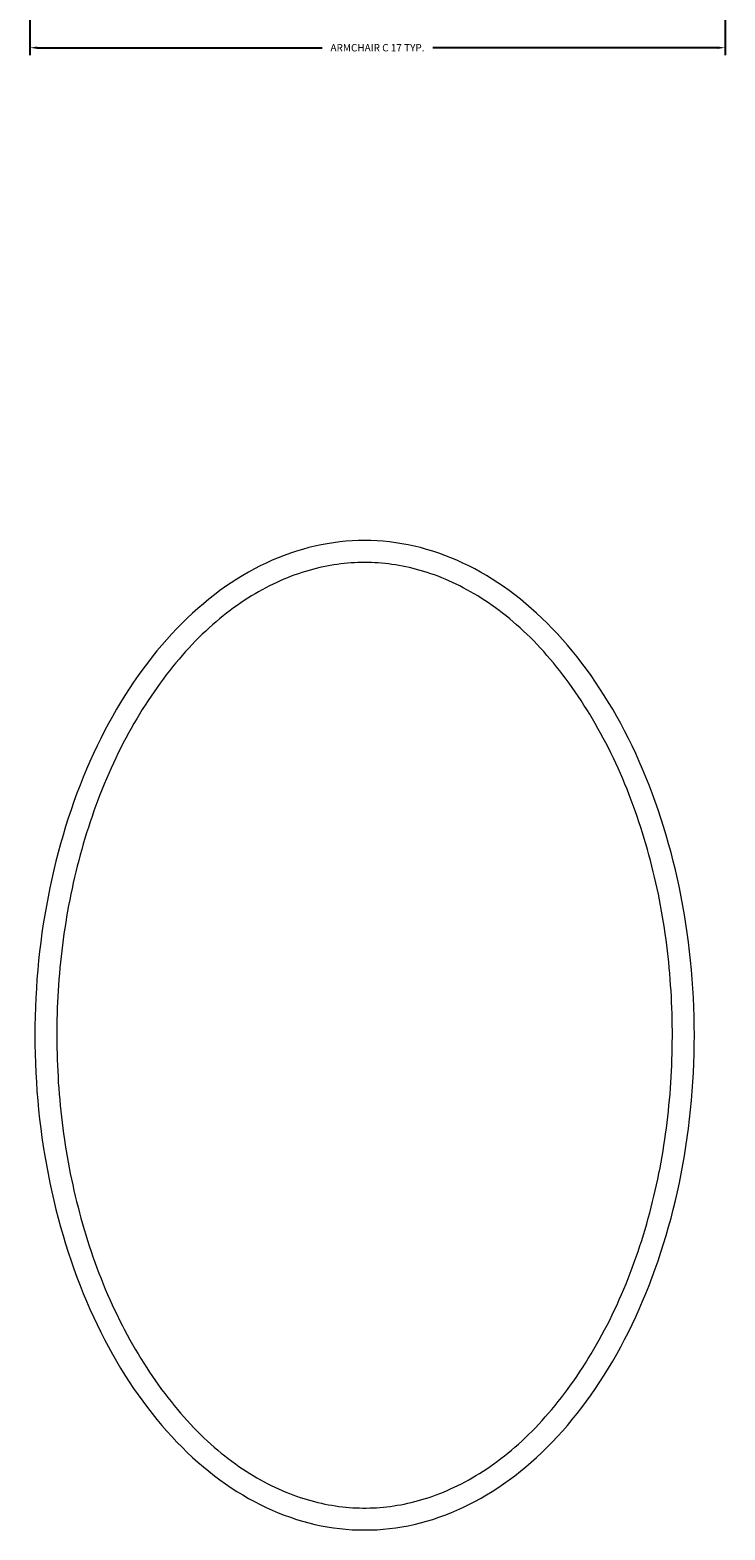
# Model space of a CAD drawing. Units: inches. Extents: x 963 to 2075, y 289 to 2657.
# Tile 22 of 98: x 1467 to 1484, y 1764 to 1800. Entities that reach past the tile are written whole.
import ezdxf

# ---------------------------------------------------------------- set-up
doc = ezdxf.new("R2010")
doc.units = ezdxf.units.IN
doc.layers.add('A-ANNO-DIMS', color=2, linetype='Continuous', lineweight=18)
doc.layers.add('A-FURN', color=8, linetype='Continuous', lineweight=18)
doc.styles.get("Standard").update_dxf_attribs({"font": 'arial.ttf'})
doc.dimstyles.get("Standard").update_dxf_attribs({"dimtxt": 0.18, "dimasz": 0.18, "dimexe": 0.18, "dimexo": 0.0625, "dimgap": 0.09, "dimtad": 0, "dimtih": 1, "dimtoh": 1, "dimdec": 4, "dimzin": 0, "dimdsep": 46, "dimtxsty": 'Standard', "dimcen": 0.09, "dimadec": 0, "dimazin": 0, "dimtfac": 1, "dimtdec": 4, "dimtofl": 0, "dimtmove": 0, "dimatfit": 3, "dimfxl": 1, "dimtolj": 1, "dimtzin": 0, "dimarcsym": 0})

# ---------------------------------------------------------------- blocks, each defined once
blk = doc.blocks.new('TABLE-OVAL')
at = {"ltscale": 0.03}
blk.add_polyline3d([(7.656, -0.197, 0), (7.809, -0.194, 0), (7.963, -0.188, 0), (8.116, -0.177, 0), (8.269, -0.162, 0), (8.422, -0.142, 0), (8.575, -0.118, 0), (8.727, -0.09, 0), (8.879, -0.057, 0), (9.031, -0.021, 0), (9.182, 0.021, 0), (9.332, 0.066, 0), (9.482, 0.116, 0), (9.632, 0.17, 0), (9.78, 0.228, 0), (9.928, 0.29, 0), (10.075, 0.357, 0), (10.221, 0.428, 0), (10.366, 0.503, 0), (10.51, 0.582, 0), (10.653, 0.665, 0), (10.796, 0.752, 0), (10.937, 0.843, 0), (11.076, 0.938, 0), (11.215, 1.037, 0), (11.352, 1.14, 0), (11.488, 1.247, 0), (11.623, 1.358, 0), (11.756, 1.472, 0), (11.888, 1.59, 0), (12.018, 1.712, 0), (12.147, 1.838, 0), (12.274, 1.967, 0), (12.399, 2.1, 0), (12.523, 2.237, 0), (12.645, 2.376, 0), (12.765, 2.52, 0), (12.883, 2.666, 0), (13, 2.817, 0), (13.114, 2.97, 0), (13.227, 3.126, 0), (13.337, 3.286, 0), (13.446, 3.449, 0), (13.552, 3.615, 0), (13.657, 3.784, 0), (13.759, 3.955, 0), (13.859, 4.13, 0), (13.957, 4.308, 0), (14.052, 4.488, 0), (14.145, 4.671, 0), (14.236, 4.856, 0), (14.325, 5.044, 0), (14.411, 5.235, 0), (14.495, 5.428, 0), (14.576, 5.623, 0), (14.655, 5.821, 0), (14.731, 6.021, 0), (14.805, 6.222, 0), (14.877, 6.426, 0), (14.945, 6.632, 0), (15.011, 6.84, 0), (15.075, 7.05, 0), (15.135, 7.261, 0), (15.193, 7.475, 0), (15.249, 7.689, 0), (15.301, 7.906, 0), (15.351, 8.123, 0), (15.399, 8.343, 0), (15.443, 8.563, 0), (15.485, 8.785, 0), (15.523, 9.007, 0), (15.559, 9.231, 0), (15.592, 9.456, 0), (15.623, 9.682, 0), (15.65, 9.908, 0), (15.675, 10.136, 0), (15.697, 10.364, 0), (15.715, 10.592, 0), (15.731, 10.821, 0), (15.744, 11.051, 0), (15.755, 11.28, 0), (15.762, 11.51, 0), (15.766, 11.741, 0), (15.768, 11.971, 0), (15.766, 12.201, 0), (15.762, 12.431, 0), (15.755, 12.661, 0), (15.744, 12.891, 0), (15.731, 13.12, 0), (15.715, 13.349, 0), (15.697, 13.578, 0), (15.675, 13.806, 0), (15.65, 14.033, 0), (15.623, 14.26, 0), (15.592, 14.486, 0), (15.559, 14.71, 0), (15.523, 14.934, 0), (15.485, 15.157, 0), (15.443, 15.379, 0), (15.399, 15.599, 0), (15.351, 15.818, 0), (15.301, 16.036, 0), (15.249, 16.252, 0), (15.193, 16.467, 0), (15.135, 16.68, 0), (15.075, 16.892, 0), (15.011, 17.101, 0), (14.945, 17.309, 0), (14.877, 17.515, 0), (14.805, 17.719, 0), (14.731, 17.921, 0), (14.655, 18.121, 0), (14.576, 18.318, 0), (14.495, 18.514, 0), (14.411, 18.707, 0), (14.325, 18.897, 0), (14.236, 19.085, 0), (14.145, 19.271, 0), (14.052, 19.454, 0), (13.957, 19.634, 0), (13.859, 19.811, 0), (13.759, 19.986, 0), (13.657, 20.158, 0), (13.552, 20.327, 0), (13.446, 20.493, 0), (13.337, 20.656, 0), (13.227, 20.815, 0), (13.114, 20.972, 0), (13, 21.125, 0), (12.883, 21.275, 0), (12.765, 21.422, 0), (12.645, 21.565, 0), (12.523, 21.705, 0), (12.399, 21.842, 0), (12.274, 21.974, 0), (12.147, 22.104, 0), (12.018, 22.229, 0), (11.888, 22.351, 0), (11.756, 22.47, 0), (11.623, 22.584, 0), (11.488, 22.695, 0), (11.352, 22.802, 0), (11.215, 22.905, 0), (11.076, 23.004, 0), (10.937, 23.099, 0), (10.796, 23.19, 0), (10.653, 23.277, 0), (10.51, 23.36, 0), (10.366, 23.439, 0), (10.221, 23.514, 0), (10.075, 23.585, 0), (9.928, 23.651, 0), (9.78, 23.714, 0), (9.632, 23.772, 0), (9.482, 23.826, 0), (9.332, 23.876, 0), (9.182, 23.921, 0), (9.031, 23.962, 0), (8.879, 23.999, 0), (8.727, 24.032, 0), (8.575, 24.06, 0), (8.422, 24.084, 0), (8.269, 24.103, 0), (8.116, 24.119, 0), (7.963, 24.13, 0), (7.809, 24.136, 0), (7.656, 24.138, 0), (7.502, 24.136, 0), (7.349, 24.13, 0), (7.196, 24.119, 0), (7.042, 24.103, 0), (6.89, 24.084, 0), (6.737, 24.06, 0), (6.585, 24.032, 0), (6.433, 23.999, 0), (6.281, 23.962, 0), (6.13, 23.921, 0), (5.979, 23.876, 0), (5.83, 23.826, 0), (5.68, 23.772, 0), (5.532, 23.714, 0), (5.384, 23.651, 0), (5.237, 23.585, 0), (5.091, 23.514, 0), (4.946, 23.439, 0), (4.802, 23.36, 0), (4.658, 23.277, 0), (4.516, 23.19, 0), (4.375, 23.099, 0), (4.236, 23.004, 0), (4.097, 22.905, 0), (3.96, 22.802, 0), (3.824, 22.695, 0), (3.689, 22.584, 0), (3.556, 22.47, 0), (3.424, 22.351, 0), (3.294, 22.229, 0), (3.165, 22.104, 0), (3.038, 21.974, 0), (2.913, 21.842, 0), (2.789, 21.705, 0), (2.667, 21.565, 0), (2.547, 21.422, 0), (2.429, 21.275, 0), (2.312, 21.125, 0), (2.198, 20.972, 0), (2.085, 20.815, 0), (1.975, 20.656, 0), (1.866, 20.493, 0), (1.76, 20.327, 0), (1.655, 20.158, 0), (1.553, 19.986, 0), (1.453, 19.811, 0), (1.355, 19.634, 0), (1.26, 19.454, 0), (1.166, 19.271, 0), (1.076, 19.085, 0), (0.987, 18.897, 0), (0.901, 18.707, 0), (0.817, 18.514, 0), (0.736, 18.318, 0), (0.657, 18.121, 0), (0.58, 17.921, 0), (0.507, 17.719, 0), (0.435, 17.515, 0), (0.367, 17.309, 0), (0.301, 17.101, 0), (0.237, 16.892, 0), (0.177, 16.68, 0), (0.118, 16.467, 0), (0.063, 16.252, 0), (0.01, 16.036, 0), (-0.039, 15.818, 0), (-0.087, 15.599, 0), (-0.131, 15.379, 0), (-0.173, 15.157, 0), (-0.211, 14.934, 0), (-0.247, 14.71, 0), (-0.281, 14.486, 0), (-0.311, 14.26, 0), (-0.338, 14.033, 0), (-0.363, 13.806, 0), (-0.385, 13.578, 0), (-0.403, 13.349, 0), (-0.419, 13.12, 0), (-0.432, 12.891, 0), (-0.443, 12.661, 0), (-0.45, 12.431, 0), (-0.454, 12.201, 0), (-0.456, 11.971, 0), (-0.454, 11.741, 0), (-0.45, 11.51, 0), (-0.443, 11.28, 0), (-0.432, 11.051, 0), (-0.419, 10.821, 0), (-0.403, 10.592, 0), (-0.385, 10.364, 0), (-0.363, 10.136, 0), (-0.338, 9.908, 0), (-0.311, 9.682, 0), (-0.281, 9.456, 0), (-0.247, 9.231, 0), (-0.211, 9.007, 0), (-0.173, 8.785, 0), (-0.131, 8.563, 0), (-0.087, 8.343, 0), (-0.039, 8.123, 0), (0.01, 7.906, 0), (0.063, 7.689, 0), (0.118, 7.475, 0), (0.177, 7.261, 0), (0.237, 7.05, 0), (0.301, 6.84, 0), (0.367, 6.632, 0), (0.435, 6.426, 0), (0.507, 6.222, 0), (0.58, 6.021, 0), (0.657, 5.821, 0), (0.736, 5.623, 0), (0.817, 5.428, 0), (0.901, 5.235, 0), (0.987, 5.044, 0), (1.076, 4.856, 0), (1.166, 4.671, 0), (1.26, 4.488, 0), (1.355, 4.308, 0), (1.453, 4.13, 0), (1.553, 3.955, 0), (1.655, 3.784, 0), (1.76, 3.615, 0), (1.866, 3.449, 0), (1.975, 3.286, 0), (2.085, 3.126, 0), (2.198, 2.97, 0), (2.312, 2.817, 0), (2.429, 2.666, 0), (2.547, 2.52, 0), (2.667, 2.376, 0), (2.789, 2.237, 0), (2.913, 2.1, 0), (3.038, 1.967, 0), (3.165, 1.838, 0), (3.294, 1.712, 0), (3.424, 1.59, 0), (3.556, 1.472, 0), (3.689, 1.358, 0), (3.824, 1.247, 0), (3.96, 1.14, 0), (4.097, 1.037, 0), (4.236, 0.938, 0), (4.375, 0.843, 0), (4.516, 0.752, 0), (4.658, 0.665, 0), (4.802, 0.582, 0), (4.946, 0.503, 0), (5.091, 0.428, 0), (5.237, 0.357, 0), (5.384, 0.29, 0), (5.532, 0.228, 0), (5.68, 0.17, 0), (5.83, 0.116, 0), (5.979, 0.066, 0), (6.13, 0.021, 0), (6.281, -0.021, 0), (6.433, -0.057, 0), (6.585, -0.09, 0), (6.737, -0.118, 0), (6.89, -0.142, 0), (7.042, -0.162, 0), (7.196, -0.177, 0), (7.349, -0.188, 0), (7.502, -0.194, 0), (7.656, -0.197, 0)], dxfattribs=at)
blk.add_polyline3d([(7.656, 0.344, 0), (7.739, 0.345, 0), (7.822, 0.347, 0), (7.906, 0.351, 0), (7.99, 0.356, 0), (8.074, 0.362, 0), (8.159, 0.37, 0), (8.244, 0.38, 0), (8.33, 0.391, 0), (8.415, 0.404, 0), (8.501, 0.418, 0), (8.588, 0.434, 0), (8.674, 0.451, 0), (8.761, 0.47, 0), (8.848, 0.491, 0), (8.935, 0.513, 0), (9.023, 0.538, 0), (9.11, 0.563, 0), (9.198, 0.591, 0), (9.286, 0.62, 0), (9.375, 0.651, 0), (9.463, 0.684, 0), (9.552, 0.719, 0), (9.64, 0.755, 0), (9.729, 0.794, 0), (9.818, 0.834, 0), (9.907, 0.876, 0), (9.995, 0.92, 0), (10.084, 0.966, 0), (10.173, 1.013, 0), (10.262, 1.063, 0), (10.35, 1.114, 0), (10.439, 1.167, 0), (10.527, 1.222, 0), (10.615, 1.279, 0), (10.703, 1.338, 0), (10.791, 1.398, 0), (10.878, 1.461, 0), (10.965, 1.525, 0), (11.052, 1.592, 0), (11.139, 1.66, 0), (11.225, 1.73, 0), (11.311, 1.802, 0), (11.396, 1.876, 0), (11.481, 1.952, 0), (11.565, 2.03, 0), (11.649, 2.109, 0), (11.733, 2.191, 0), (11.815, 2.275, 0), (11.898, 2.361, 0), (11.98, 2.448, 0), (12.061, 2.537, 0), (12.141, 2.629, 0), (12.221, 2.721, 0), (12.301, 2.816, 0), (12.379, 2.912, 0), (12.457, 3.01, 0), (12.535, 3.11, 0), (12.611, 3.211, 0), (12.687, 3.314, 0), (12.762, 3.418, 0), (12.836, 3.524, 0), (12.909, 3.632, 0), (12.982, 3.741, 0), (13.053, 3.851, 0), (13.124, 3.963, 0), (13.194, 4.076, 0), (13.262, 4.191, 0), (13.33, 4.307, 0), (13.397, 4.424, 0), (13.463, 4.543, 0), (13.528, 4.662, 0), (13.591, 4.783, 0), (13.654, 4.906, 0), (13.716, 5.029, 0), (13.776, 5.154, 0), (13.835, 5.279, 0), (13.893, 5.406, 0), (13.95, 5.534, 0), (14.006, 5.663, 0), (14.061, 5.792, 0), (14.114, 5.923, 0), (14.166, 6.055, 0), (14.217, 6.188, 0), (14.266, 6.321, 0), (14.314, 6.455, 0), (14.361, 6.589, 0), (14.406, 6.723, 0), (14.45, 6.858, 0), (14.493, 6.993, 0), (14.535, 7.129, 0), (14.575, 7.265, 0), (14.614, 7.401, 0), (14.652, 7.537, 0), (14.688, 7.674, 0), (14.724, 7.811, 0), (14.758, 7.948, 0), (14.791, 8.086, 0), (14.822, 8.223, 0), (14.852, 8.361, 0), (14.882, 8.5, 0), (14.909, 8.638, 0), (14.936, 8.777, 0), (14.961, 8.916, 0), (14.986, 9.055, 0), (15.009, 9.194, 0), (15.031, 9.334, 0), (15.051, 9.473, 0), (15.071, 9.613, 0), (15.089, 9.753, 0), (15.106, 9.893, 0), (15.122, 10.033, 0), (15.137, 10.174, 0), (15.151, 10.314, 0), (15.163, 10.455, 0), (15.175, 10.596, 0), (15.185, 10.736, 0), (15.194, 10.877, 0), (15.202, 11.018, 0), (15.209, 11.159, 0), (15.215, 11.3, 0), (15.219, 11.441, 0), (15.223, 11.583, 0), (15.225, 11.724, 0), (15.227, 11.865, 0), (15.227, 12.006, 0), (15.226, 12.147, 0), (15.224, 12.288, 0), (15.221, 12.43, 0), (15.217, 12.571, 0), (15.212, 12.712, 0), (15.205, 12.853, 0), (15.198, 12.994, 0), (15.19, 13.135, 0), (15.18, 13.276, 0), (15.169, 13.416, 0), (15.157, 13.557, 0), (15.144, 13.698, 0), (15.13, 13.838, 0), (15.114, 13.978, 0), (15.098, 14.119, 0), (15.08, 14.259, 0), (15.061, 14.399, 0), (15.041, 14.538, 0), (15.02, 14.678, 0), (14.997, 14.817, 0), (14.974, 14.956, 0), (14.949, 15.095, 0), (14.923, 15.234, 0), (14.896, 15.373, 0), (14.867, 15.511, 0), (14.837, 15.649, 0), (14.806, 15.787, 0), (14.774, 15.925, 0), (14.741, 16.062, 0), (14.706, 16.199, 0), (14.67, 16.336, 0), (14.633, 16.473, 0), (14.595, 16.609, 0), (14.555, 16.745, 0), (14.514, 16.881, 0), (14.472, 17.016, 0), (14.428, 17.151, 0), (14.384, 17.286, 0), (14.338, 17.42, 0), (14.29, 17.554, 0), (14.241, 17.687, 0), (14.191, 17.821, 0), (14.14, 17.953, 0), (14.087, 18.084, 0), (14.034, 18.214, 0), (13.978, 18.344, 0), (13.922, 18.472, 0), (13.865, 18.599, 0), (13.806, 18.725, 0), (13.746, 18.85, 0), (13.685, 18.974, 0), (13.623, 19.097, 0), (13.56, 19.219, 0), (13.495, 19.339, 0), (13.43, 19.458, 0), (13.364, 19.576, 0), (13.296, 19.693, 0), (13.228, 19.808, 0), (13.159, 19.922, 0), (13.089, 20.035, 0), (13.017, 20.146, 0), (12.945, 20.255, 0), (12.873, 20.364, 0), (12.799, 20.47, 0), (12.724, 20.576, 0), (12.649, 20.679, 0), (12.573, 20.781, 0), (12.496, 20.882, 0), (12.418, 20.981, 0), (12.34, 21.078, 0), (12.261, 21.173, 0), (12.182, 21.267, 0), (12.101, 21.359, 0), (12.02, 21.449, 0), (11.939, 21.537, 0), (11.857, 21.624, 0), (11.774, 21.709, 0), (11.691, 21.791, 0), (11.607, 21.872, 0), (11.523, 21.951, 0), (11.438, 22.028, 0), (11.353, 22.103, 0), (11.268, 22.176, 0), (11.182, 22.247, 0), (11.095, 22.316, 0), (11.009, 22.383, 0), (10.922, 22.449, 0), (10.835, 22.512, 0), (10.747, 22.574, 0), (10.659, 22.633, 0), (10.571, 22.691, 0), (10.483, 22.747, 0), (10.395, 22.801, 0), (10.306, 22.854, 0), (10.217, 22.904, 0), (10.129, 22.952, 0), (10.04, 22.999, 0), (9.951, 23.044, 0), (9.862, 23.087, 0), (9.773, 23.128, 0), (9.685, 23.167, 0), (9.596, 23.205, 0), (9.507, 23.24, 0), (9.419, 23.274, 0), (9.331, 23.306, 0), (9.242, 23.336, 0), (9.154, 23.365, 0), (9.067, 23.391, 0), (8.979, 23.416, 0), (8.892, 23.44, 0), (8.804, 23.461, 0), (8.718, 23.481, 0), (8.631, 23.499, 0), (8.544, 23.516, 0), (8.458, 23.531, 0), (8.373, 23.545, 0), (8.287, 23.557, 0), (8.202, 23.567, 0), (8.117, 23.576, 0), (8.032, 23.583, 0), (7.948, 23.589, 0), (7.864, 23.593, 0), (7.781, 23.596, 0), (7.697, 23.597, 0), (7.615, 23.597, 0), (7.531, 23.596, 0), (7.448, 23.593, 0), (7.364, 23.589, 0), (7.28, 23.583, 0), (7.195, 23.576, 0), (7.11, 23.567, 0), (7.025, 23.557, 0), (6.939, 23.545, 0), (6.854, 23.531, 0), (6.767, 23.516, 0), (6.681, 23.499, 0), (6.594, 23.481, 0), (6.507, 23.461, 0), (6.42, 23.44, 0), (6.333, 23.416, 0), (6.245, 23.391, 0), (6.158, 23.365, 0), (6.07, 23.336, 0), (5.981, 23.306, 0), (5.893, 23.274, 0), (5.805, 23.24, 0), (5.716, 23.205, 0), (5.627, 23.167, 0), (5.539, 23.128, 0), (5.45, 23.087, 0), (5.361, 23.044, 0), (5.272, 22.999, 0), (5.183, 22.952, 0), (5.095, 22.904, 0), (5.006, 22.854, 0), (4.917, 22.801, 0), (4.829, 22.747, 0), (4.741, 22.691, 0), (4.653, 22.633, 0), (4.565, 22.574, 0), (4.477, 22.512, 0), (4.39, 22.449, 0), (4.303, 22.383, 0), (4.216, 22.316, 0), (4.13, 22.247, 0), (4.044, 22.176, 0), (3.959, 22.103, 0), (3.874, 22.028, 0), (3.789, 21.951, 0), (3.705, 21.872, 0), (3.621, 21.791, 0), (3.538, 21.709, 0), (3.455, 21.624, 0), (3.373, 21.537, 0), (3.292, 21.449, 0), (3.211, 21.359, 0), (3.13, 21.267, 0), (3.051, 21.173, 0), (2.972, 21.078, 0), (2.893, 20.981, 0), (2.816, 20.882, 0), (2.739, 20.781, 0), (2.663, 20.679, 0), (2.588, 20.576, 0), (2.513, 20.47, 0), (2.439, 20.364, 0), (2.366, 20.255, 0), (2.294, 20.146, 0), (2.223, 20.035, 0), (2.153, 19.922, 0), (2.084, 19.808, 0), (2.016, 19.693, 0), (1.948, 19.576, 0), (1.882, 19.458, 0), (1.817, 19.339, 0), (1.752, 19.219, 0), (1.689, 19.097, 0), (1.627, 18.974, 0), (1.566, 18.85, 0), (1.506, 18.725, 0), (1.447, 18.599, 0), (1.39, 18.472, 0), (1.334, 18.344, 0), (1.278, 18.214, 0), (1.225, 18.084, 0), (1.172, 17.953, 0), (1.121, 17.821, 0), (1.071, 17.687, 0), (1.022, 17.554, 0), (0.974, 17.42, 0), (0.928, 17.286, 0), (0.884, 17.151, 0), (0.84, 17.016, 0), (0.798, 16.881, 0), (0.757, 16.745, 0), (0.717, 16.609, 0), (0.679, 16.473, 0), (0.642, 16.336, 0), (0.606, 16.199, 0), (0.571, 16.062, 0), (0.538, 15.925, 0), (0.505, 15.787, 0), (0.475, 15.649, 0), (0.445, 15.511, 0), (0.416, 15.373, 0), (0.389, 15.234, 0), (0.363, 15.095, 0), (0.338, 14.956, 0), (0.315, 14.817, 0), (0.292, 14.678, 0), (0.271, 14.538, 0), (0.251, 14.399, 0), (0.232, 14.259, 0), (0.214, 14.119, 0), (0.198, 13.978, 0), (0.182, 13.838, 0), (0.168, 13.698, 0), (0.155, 13.557, 0), (0.143, 13.416, 0), (0.132, 13.276, 0), (0.122, 13.135, 0), (0.114, 12.994, 0), (0.106, 12.853, 0), (0.1, 12.712, 0), (0.095, 12.571, 0), (0.091, 12.43, 0), (0.088, 12.288, 0), (0.086, 12.147, 0), (0.085, 12.006, 0), (0.085, 11.865, 0), (0.087, 11.724, 0), (0.089, 11.583, 0), (0.093, 11.441, 0), (0.097, 11.3, 0), (0.103, 11.159, 0), (0.11, 11.018, 0), (0.118, 10.877, 0), (0.127, 10.736, 0), (0.137, 10.596, 0), (0.149, 10.455, 0), (0.161, 10.314, 0), (0.175, 10.174, 0), (0.19, 10.033, 0), (0.206, 9.893, 0), (0.223, 9.753, 0), (0.241, 9.613, 0), (0.261, 9.473, 0), (0.281, 9.334, 0), (0.303, 9.194, 0), (0.326, 9.055, 0), (0.35, 8.916, 0), (0.376, 8.777, 0), (0.403, 8.638, 0), (0.43, 8.5, 0), (0.46, 8.361, 0), (0.49, 8.223, 0), (0.521, 8.086, 0), (0.554, 7.948, 0), (0.588, 7.811, 0), (0.623, 7.674, 0), (0.66, 7.537, 0), (0.698, 7.401, 0), (0.737, 7.265, 0), (0.777, 7.129, 0), (0.819, 6.993, 0), (0.862, 6.858, 0), (0.906, 6.723, 0), (0.951, 6.589, 0), (0.998, 6.455, 0), (1.046, 6.321, 0), (1.095, 6.188, 0), (1.146, 6.055, 0), (1.198, 5.923, 0), (1.251, 5.792, 0), (1.306, 5.663, 0), (1.362, 5.534, 0), (1.418, 5.406, 0), (1.477, 5.279, 0), (1.536, 5.154, 0), (1.596, 5.029, 0), (1.658, 4.906, 0), (1.721, 4.783, 0), (1.784, 4.662, 0), (1.849, 4.543, 0), (1.915, 4.424, 0), (1.982, 4.307, 0), (2.05, 4.191, 0), (2.118, 4.076, 0), (2.188, 3.963, 0), (2.259, 3.851, 0), (2.33, 3.741, 0), (2.403, 3.632, 0), (2.476, 3.524, 0), (2.55, 3.418, 0), (2.625, 3.314, 0), (2.701, 3.211, 0), (2.777, 3.11, 0), (2.855, 3.01, 0), (2.933, 2.912, 0), (3.011, 2.816, 0), (3.09, 2.721, 0), (3.17, 2.629, 0), (3.251, 2.537, 0), (3.332, 2.448, 0), (3.414, 2.361, 0), (3.497, 2.275, 0), (3.579, 2.191, 0), (3.663, 2.109, 0), (3.747, 2.03, 0), (3.831, 1.952, 0), (3.916, 1.876, 0), (4.001, 1.802, 0), (4.087, 1.73, 0), (4.173, 1.66, 0), (4.26, 1.592, 0), (4.347, 1.525, 0), (4.434, 1.461, 0), (4.521, 1.398, 0), (4.609, 1.338, 0), (4.697, 1.279, 0), (4.785, 1.222, 0), (4.873, 1.167, 0), (4.962, 1.114, 0), (5.05, 1.063, 0), (5.139, 1.013, 0), (5.228, 0.966, 0), (5.316, 0.92, 0), (5.405, 0.876, 0), (5.494, 0.834, 0), (5.583, 0.794, 0), (5.672, 0.755, 0), (5.76, 0.719, 0), (5.849, 0.684, 0), (5.937, 0.651, 0), (6.026, 0.62, 0), (6.114, 0.591, 0), (6.201, 0.563, 0), (6.289, 0.538, 0), (6.377, 0.513, 0), (6.464, 0.491, 0), (6.551, 0.47, 0), (6.638, 0.451, 0), (6.724, 0.434, 0), (6.811, 0.418, 0), (6.897, 0.404, 0), (6.982, 0.391, 0), (7.068, 0.38, 0), (7.153, 0.37, 0), (7.237, 0.362, 0), (7.322, 0.356, 0), (7.406, 0.351, 0), (7.49, 0.347, 0), (7.573, 0.345, 0), (7.656, 0.344, 0)])
blk = doc.blocks.new('*D26')
at = {"layer": 'A-ANNO-DIMS', "color": 0, "lineweight": -2, "transparency": 16777216}
for p, q in [((1467.146, 1802.491), (1467.146, 1799.809)), ((1484.243, 1802.491), (1484.243, 1799.809)), ((1467.326, 1799.989), (1474.33, 1799.989)), ((1484.063, 1799.989), (1477.059, 1799.989))]:
    blk.add_line(p, q, dxfattribs=at)
at = {"layer": 'A-ANNO-DIMS', "color": 0, "transparency": 16777216}
for points in [[(1467.326, 1800.019), (1467.326, 1799.959), (1467.146, 1799.989)], [(1484.063, 1800.019), (1484.063, 1799.959), (1484.243, 1799.989)]]:
    blk.add_solid(points, dxfattribs=at)
at = {"layer": 'Defpoints', "color": 0, "transparency": 16777216}
for p in [(1467.146, 1802.554), (1484.243, 1802.554), (1484.243, 1799.989)]:
    blk.add_point(p, dxfattribs=at)
at = {"layer": 'A-ANNO-DIMS', "color": 0, "transparency": 16777216, "insert": (1475.694, 1799.989), "char_height": 0.18, "attachment_point": 5}
blk.add_mtext('\\A1;ARMCHAIR C 17 TYP.', dxfattribs=at)

msp = doc.modelspace()

# ---------------------------------------------------------------- block references
at = {"layer": 'A-FURN', "rotation": 180}
msp.add_blockref('TABLE-OVAL', (1483.033, 1787.674), dxfattribs=at)

# ---------------------------------------------------------------- dimensions: what is measured, and where the dimension line sits
at = {"layer": 'A-ANNO-DIMS'}
dim = msp.add_linear_dim(base=(1484.243, 1799.989), p1=(1467.146, 1802.554), p2=(1484.243, 1802.554), text='ARMCHAIR C <> TYP.', dimstyle='Standard', override={"dimdec": 0, "dimlfac": 1, "dimrnd": 0, "dimzin": 0, "dimdsep": 46, "dimlunit": 2}, dxfattribs=at)
dim.commit()
dim.dimension.update_dxf_attribs({"geometry": '*D26', "text_midpoint": (1475.694, 1799.989)})

doc.saveas('drawing.dxf')
